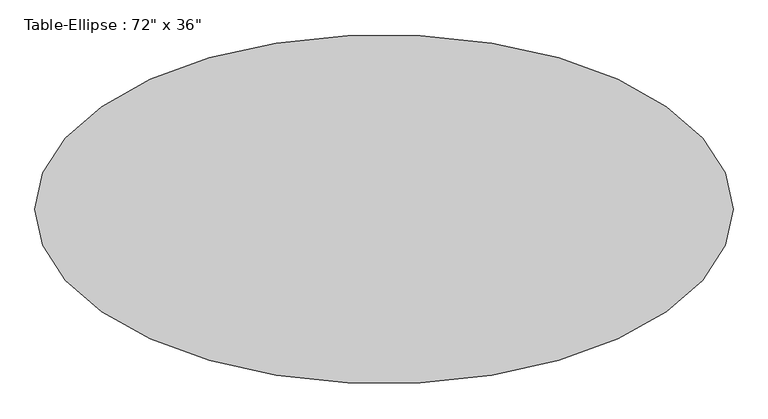
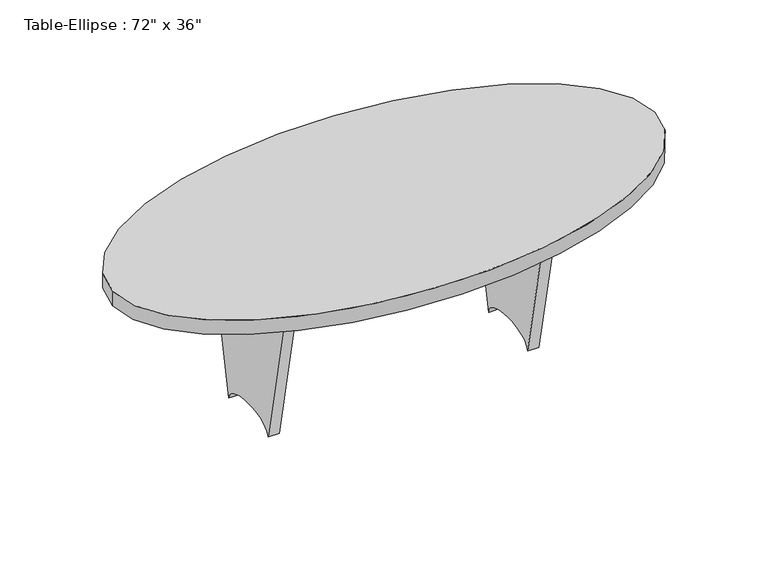
"""IFC4 building model written with IfcOpenShell, lengths in millimetres: furniture geometry."""

from ifc_helpers import new_model, si_unit, point, frame, origin, place, context, project, spatial, ellipse_curve, trimmed, source, transform, mapped, element, save
from ifc_brep_helpers import plane_surface, extruded_surface, advanced_brep


def furniture_c045eb45(model_context):
    return source(origin(), model_context, "Body", "AdvancedBrep", [
        advanced_brep(
        [(-914.4, 0.0, 609.6), (914.4, 0.0, 609.6), (-914.4, 0.0, 558.8), (914.4, 0.0, 558.8)],
        [
            (0, 1, ellipse_curve(frame((0.0, 0.0, 609.6), z_axis=(0.0, 0.0, 1.0), x_axis=(1.0, 0.0, 0.0)), 914.4, 457.2)),
            (1, 0, ellipse_curve(frame((0.0, 0.0, 609.6), z_axis=(0.0, 0.0, 1.0), x_axis=(1.0, 0.0, 0.0)), 914.4, 457.2)),
            (2, 3, ellipse_curve(frame((0.0, 0.0, 558.8), z_axis=(0.0, 0.0, -1.0), x_axis=(1.0, 0.0, 0.0)), 914.4, 457.2)),
            (3, 2, ellipse_curve(frame((0.0, 0.0, 558.8), z_axis=(0.0, 0.0, -1.0), x_axis=(1.0, 0.0, 0.0)), 914.4, 457.2)),
            (0, 2),
            (3, 1),
        ],
        [
            plane_surface(frame((914.4, 0.0, 609.6), z_axis=(0.0, 0.0, 1.0), x_axis=(0.0, 1.0, 0.0))),
            plane_surface(frame((914.4, 0.0, 558.8), z_axis=(0.0, 0.0, -1.0), x_axis=(0.0, -1.0, 0.0))),
            extruded_surface(trimmed(ellipse_curve(frame((0.0, 0.0, 508.0), z_axis=(0.0, 0.0, 1.0), x_axis=(1.0, 0.0, 0.0)), 914.4, 457.2), [point((-914.4, 0.0, 508.0))], [point((914.4, 0.0, 508.0))], True, "CARTESIAN"), (0.0, 0.0, 50.799999999999955), 50.799999999999955),
            extruded_surface(trimmed(ellipse_curve(frame((0.0, 0.0, 508.0), z_axis=(0.0, 0.0, 1.0), x_axis=(1.0, 0.0, 0.0)), 914.4, 457.2), [point((914.4, 0.0, 508.0))], [point((-914.4, 0.0, 508.0))], True, "CARTESIAN"), (0.0, 0.0, 50.799999999999955), 50.799999999999955),
        ],
        [
            (0, [[1, 2]]),
            (1, [[3, 4]]),
            (2, [[-1, 5, -4, 6]]),
            (3, [[-2, -6, -3, -5]]),
        ],
    ),
        advanced_brep(
        [(-419.1, 228.6, 558.8), (-419.1, -228.6, 558.8), (-419.1, -114.3, 0.0), (-419.1, 114.3, 0.0), (-457.2, 228.6, 558.8), (-457.2, 114.3, 0.0), (-457.2, -114.3, 0.0), (-457.2, -228.6, 558.8)],
        [
            (0, 1),
            (1, 2),
            (2, 3, ellipse_curve(frame((-419.1, 0.0, 0.0), z_axis=(-1.0, 0.0, 0.0), x_axis=(0.0, 1.0, 0.0)), 114.3, 50.8)),
            (3, 0),
            (4, 5),
            (5, 6, ellipse_curve(frame((-457.2, 0.0, 0.0), z_axis=(1.0, 0.0, 0.0), x_axis=(0.0, 1.0, 0.0)), 114.3, 50.8)),
            (6, 7),
            (7, 4),
            (0, 4),
            (7, 1),
            (6, 2),
            (5, 3),
        ],
        [
            plane_surface(frame((-419.1, -228.6, 558.8), z_axis=(1.0, 0.0, 0.0), x_axis=(0.0, -1.0, 0.0))),
            plane_surface(frame((-457.2, -228.6, 558.8), z_axis=(-1.0, 0.0, 0.0), x_axis=(0.0, 1.0, 0.0))),
            plane_surface(frame((-419.1, 228.6, 558.8), z_axis=(0.0, 0.0, 1.0), x_axis=(-1.0, 0.0, 0.0))),
            plane_surface(frame((-419.1, -228.6, 558.8), z_axis=(0.0, -0.979714932282564, -0.20039623614871369), x_axis=(-1.0, 0.0, 0.0))),
            extruded_surface(trimmed(ellipse_curve(frame((-495.3, 0.0, 0.0), z_axis=(-1.0, 0.0, 0.0), x_axis=(0.0, 1.0, 0.0)), 114.3, 50.8), [point((-495.3, -114.3, 0.0))], [point((-495.3, 114.3, 0.0))], True, "CARTESIAN"), (38.10000000000002, 0.0, 0.0), 38.10000000000002),
            plane_surface(frame((-419.1, 114.3, 0.0), z_axis=(0.0, 0.9797149322825663, -0.2003962361487023), x_axis=(-1.0, 0.0, 0.0))),
        ],
        [
            (0, [[1, 2, 3, 4]]),
            (1, [[5, 6, 7, 8]]),
            (2, [[-1, 9, -8, 10]]),
            (3, [[-2, -10, -7, 11]]),
            (4, [[-3, -11, -6, 12]]),
            (5, [[-4, -12, -5, -9]]),
        ],
    ),
        advanced_brep(
        [(457.2, 228.6, 558.8), (457.2, -228.6, 558.8), (457.2, -114.3, 0.0), (457.2, 114.3, 0.0), (419.1, 228.6, 558.8), (419.1, 114.3, 0.0), (419.1, -114.3, 0.0), (419.1, -228.6, 558.8)],
        [
            (0, 1),
            (1, 2),
            (2, 3, ellipse_curve(frame((457.2, 0.0, 0.0), z_axis=(-1.0, 0.0, 0.0), x_axis=(0.0, 1.0, 0.0)), 114.3, 50.8)),
            (3, 0),
            (4, 5),
            (5, 6, ellipse_curve(frame((419.1, 0.0, 0.0), z_axis=(1.0, 0.0, 0.0), x_axis=(0.0, 1.0, 0.0)), 114.3, 50.8)),
            (6, 7),
            (7, 4),
            (0, 4),
            (7, 1),
            (6, 2),
            (5, 3),
        ],
        [
            plane_surface(frame((457.2, -228.6, 558.8), z_axis=(1.0, 0.0, 0.0), x_axis=(0.0, -1.0, 0.0))),
            plane_surface(frame((419.1, -228.6, 558.8), z_axis=(-1.0, 0.0, 0.0), x_axis=(0.0, 1.0, 0.0))),
            plane_surface(frame((457.2, 228.6, 558.8), z_axis=(0.0, 0.0, 1.0), x_axis=(-1.0, 0.0, 0.0))),
            plane_surface(frame((457.2, -228.6, 558.8), z_axis=(0.0, -0.9797149322825643, -0.20039623614871194), x_axis=(-1.0, 0.0, 0.0))),
            extruded_surface(trimmed(ellipse_curve(frame((381.0, 0.0, 0.0), z_axis=(-1.0, 0.0, 0.0), x_axis=(0.0, 1.0, 0.0)), 114.3, 50.8), [point((381.0, -114.3, 0.0))], [point((381.0, 114.3, 0.0))], True, "CARTESIAN"), (38.10000000000002, 0.0, 0.0), 38.10000000000002),
            plane_surface(frame((457.2, 114.3, 0.0), z_axis=(0.0, 0.979714932282567, -0.20039623614869895), x_axis=(-1.0, 0.0, 0.0))),
        ],
        [
            (0, [[1, 2, 3, 4]]),
            (1, [[5, 6, 7, 8]]),
            (2, [[-1, 9, -8, 10]]),
            (3, [[-2, -10, -7, 11]]),
            (4, [[-3, -11, -6, 12]]),
            (5, [[-4, -12, -5, -9]]),
        ],
    ),
        advanced_brep(
        [(-419.1, 19.05, 558.8), (419.1, 19.05, 558.8), (419.1, 19.05, 372.5333333), (-419.1, 19.05, 372.5333333), (-419.1, -19.05, 558.8), (-419.1, -19.05, 372.5333333), (419.1, -19.05, 372.5333333), (419.1, -19.05, 558.8)],
        [
            (0, 1),
            (1, 2),
            (2, 3, ellipse_curve(frame((0.0, 19.05, 372.5333333), z_axis=(0.0, -1.0, 0.0), x_axis=(1.0, 0.0, 0.0)), 419.1, 101.6)),
            (3, 0),
            (4, 5),
            (5, 6, ellipse_curve(frame((0.0, -19.05, 372.5333333), z_axis=(0.0, 1.0, 0.0), x_axis=(1.0, 0.0, 0.0)), 419.1, 101.6)),
            (6, 7),
            (7, 4),
            (0, 4),
            (7, 1),
            (6, 2),
            (5, 3),
        ],
        [
            plane_surface(frame((-419.1, 19.05, 558.8), z_axis=(0.0, 1.0, 0.0), x_axis=(1.0, 0.0, 0.0))),
            plane_surface(frame((-419.1, -19.05, 558.8), z_axis=(0.0, -1.0, 0.0), x_axis=(-1.0, 0.0, 0.0))),
            plane_surface(frame((-419.1, 19.05, 558.8), z_axis=(0.0, 0.0, 1.0), x_axis=(0.0, -1.0, 0.0))),
            plane_surface(frame((419.1, 19.05, 558.8), z_axis=(1.0, 0.0, 0.0), x_axis=(0.0, -1.0, 0.0))),
            extruded_surface(trimmed(ellipse_curve(frame((0.0, -57.15, 372.5333333), z_axis=(0.0, -1.0, 0.0), x_axis=(1.0, 0.0, 0.0)), 419.1, 101.6), [point((419.1, -57.15, 372.5333333))], [point((-419.1, -57.15, 372.5333333))], True, "CARTESIAN"), (0.0, 38.099999999999994, 0.0), 38.099999999999994),
            plane_surface(frame((-419.1, 19.05, 372.5333333), z_axis=(-1.0, 0.0, 0.0), x_axis=(0.0, -1.0, 0.0))),
        ],
        [
            (0, [[1, 2, 3, 4]]),
            (1, [[5, 6, 7, 8]]),
            (2, [[-1, 9, -8, 10]]),
            (3, [[-2, -10, -7, 11]]),
            (4, [[-3, -11, -6, 12]]),
            (5, [[-4, -12, -5, -9]]),
        ],
    ),
    ])


if __name__ == "__main__":
    model = new_model("IFC4")
    model_context = context("Model", 3, world=origin())
    ifc_project = project(units=[si_unit("LENGTHUNIT", "METRE", prefix="MILLI")], contexts=[model_context])
    site = spatial("IfcSite", under=ifc_project)
    building = spatial("IfcBuilding", under=site)
    placement = place(None, origin())
    furniture_shape = furniture_c045eb45(model_context)
    element("IfcFurniture", 1, ObjectType="Table-Ellipse : 72\" x 36\"", at=placement, inside=building, context=model_context, shape_type="MappedRepresentation", body=[
        mapped(furniture_shape, transform((0.0, 0.0, 0.0), x_axis=(1.0, 0.0, 0.0), y_axis=(0.0, 1.0, 0.0), z_axis=(0.0, 0.0, 1.0))),
    ])
    save(model, "model.ifc")

# Revit data of these elements
# Type "Table-Ellipse : 72\" x 36\""
#   Assembly Code = "E2020200"
#   Half Width = 1' - 6"
#   Half Length = 3' - 0"
#   Height = 2' - 0"
#   Length = 6' - 0"
#   Width = 3' - 0"
#   Base Material = Birch
#   Top Material = Laminate - Black
#   Default Elevation = 0
# Element 1 (IfcFurniture, "Table-Ellipse : 72\" x 36\"")
#   Materials on its faces: "Birch", "Laminate - Black"
# Materials
#   "Birch": class "Wood", colour RGB 224 178 126, transparency 0, Description = "Betula Alleghaniensis", Cost = 0
#   "Laminate - Black": colour RGB 0 0 0, transparency 0
